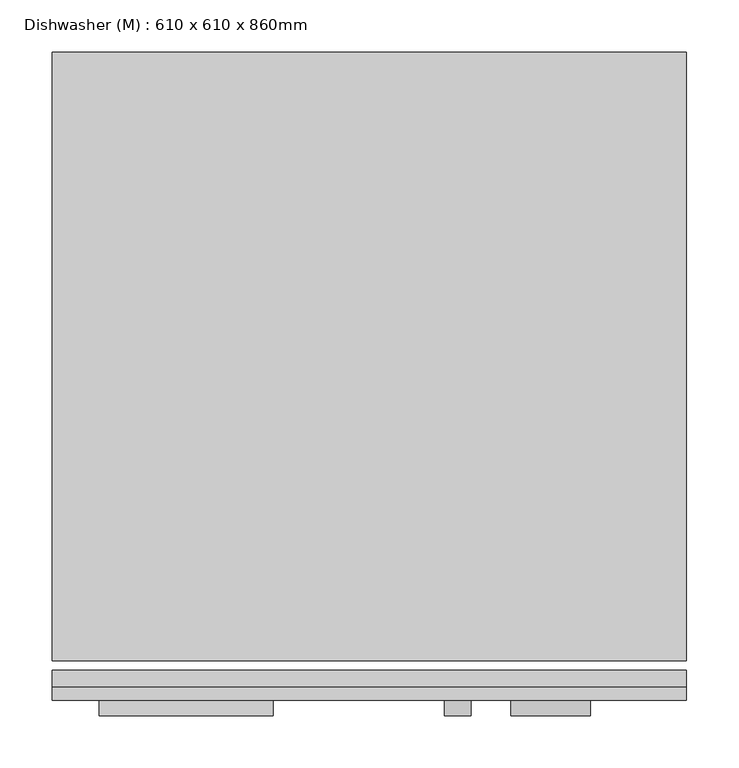
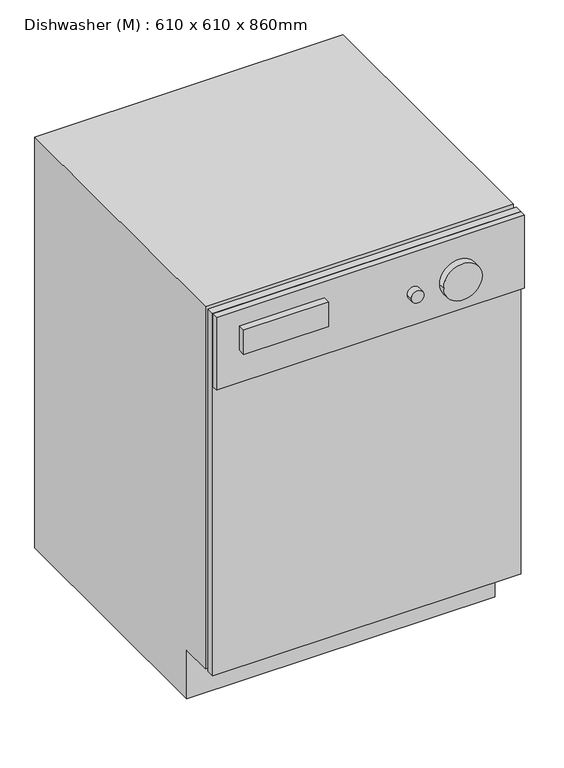
"""IFC4 building model written with IfcOpenShell, lengths in millimetres: proxy geometry, Dishwasher (M) : 610 x 610 x 860mm."""

from ifc_helpers import new_model, si_unit, point, frame, frame_2d, origin, place, context, project, spatial, polyline, circle_curve, trimmed, segment, composite_curve, outline, extrude, source, transform, mapped, element, save


def dishwasher_m_610_x_610_x_860mm_47db8dec(model_context):
    return source(origin(), model_context, "Body", "SweptSolid", [
        extrude(outline(polyline([(687.5174685, -38.3504352), (77.5174685, -38.3504352), (77.5174685, -22.4754352), (687.5174685, -22.4754352), (687.5174685, -38.3504352)])), frame((0.0, 0.0, 101.6), z_axis=(0.0, 0.0, 1.0), x_axis=(1.0, 0.0, 0.0)), (0.0, 0.0, 1.0), 758.4),
        extrude(outline(polyline([(687.5174685, -38.3504352), (687.5174685, -51.0504352), (77.5174685, -51.0504352), (77.5174685, -38.3504352), (687.5174685, -38.3504352)])), frame((0.0, 0.0, 707.6), z_axis=(0.0, 0.0, 1.0), x_axis=(1.0, 0.0, 0.0)), (0.0, 0.0, 1.0), 152.4),
        extrude(outline(polyline([(571.6495648, 0.0), (50.5495648, 0.0), (50.5495648, 101.6), (-12.9504352, 101.6), (-12.9504352, 860.0), (571.6495648, 860.0), (571.6495648, 0.0)])), frame((77.5174685, 0.0, 0.0), z_axis=(1.0, 0.0, 0.0), x_axis=(0.0, 1.0, 0.0)), (0.0, 0.0, 1.0), 610.0),
        extrude(outline(polyline([(290.2347603, -66.0504352), (122.8347603, -66.0504352), (122.8347603, -51.0504352), (290.2347603, -51.0504352), (290.2347603, -66.0504352)])), frame((0.0, 0.0, 775.6663551), z_axis=(0.0, 0.0, 1.0), x_axis=(1.0, 0.0, 0.0)), (0.0, 0.0, 1.0), 50.8),
        extrude(outline(composite_curve([segment(trimmed(circle_curve(frame_2d((775.6663551, 467.3393328)), 12.7), [point((775.6663551, 480.0393328))], [point((775.6663551, 454.6393328))], False, "CARTESIAN"), True, "CONTINUOUS"), segment(trimmed(circle_curve(frame_2d((775.6663551, 467.3393328)), 12.7), [point((775.6663551, 454.6393328))], [point((775.6663551, 480.0393328))], False, "CARTESIAN"), True, "CONTINUOUS")], self_intersect=False)), frame((0.0, -66.0504352, 0.0), z_axis=(0.0, 1.0, 0.0), x_axis=(0.0, 0.0, 1.0)), (0.0, 0.0, 1.0), 15.0),
        extrude(outline(composite_curve([segment(trimmed(circle_curve(frame_2d((775.6663551, 556.7855874)), 38.1), [point((775.6663551, 594.8855874))], [point((775.6663551, 518.6855874))], False, "CARTESIAN"), True, "CONTINUOUS"), segment(trimmed(circle_curve(frame_2d((775.6663551, 556.7855874)), 38.1), [point((775.6663551, 518.6855874))], [point((775.6663551, 594.8855874))], False, "CARTESIAN"), True, "CONTINUOUS")], self_intersect=False)), frame((0.0, -66.0504352, 0.0), z_axis=(0.0, 1.0, 0.0), x_axis=(0.0, 0.0, 1.0)), (0.0, 0.0, 1.0), 15.0),
    ])


if __name__ == "__main__":
    model = new_model("IFC4")
    model_context = context("Model", 3, world=origin())
    ifc_project = project(units=[si_unit("LENGTHUNIT", "METRE", prefix="MILLI")], contexts=[model_context])
    site = spatial("IfcSite", under=ifc_project)
    building = spatial("IfcBuilding", under=site)
    placement = place(None, origin())
    dishwasher_m_610_x_610_x_860mm_shape = dishwasher_m_610_x_610_x_860mm_47db8dec(model_context)
    element("IfcBuildingElementProxy", 1, Name="Dishwasher (M) : 610 x 610 x 860mm", ObjectType="Dishwasher (M) : 610 x 610 x 860mm", at=placement, inside=building, context=model_context, shape_type="MappedRepresentation", body=[
        mapped(dishwasher_m_610_x_610_x_860mm_shape, transform((0.0, 0.0, 0.0), x_axis=(1.0, 0.0, 0.0), y_axis=(0.0, 1.0, 0.0), z_axis=(0.0, 0.0, 1.0))),
    ])
    save(model, "model.ifc")

# Revit data of these elements
# Type "Dishwasher (M) : 610 x 610 x 860mm"
#   Label = "DW"
#   Depth = 2' - 0.01575"
#   Height = 2' - 9.85827"
#   Width = 2' - 0.01575"
#   Dishwasher Material = Metal - Paint Finish - Ivory,Glossy
#   Panel Face Material = Plastic - Black
#   Default Elevation = 0
# Element 1 (IfcBuildingElementProxy, "Dishwasher (M) : 610 x 610 x 860mm")
#   Materials on its faces: "Metal - Paint Finish - Ivory,Glossy", "Plastic - Black"
# Materials
#   "Metal - Paint Finish - Ivory,Glossy": colour RGB 247 247 239, transparency 0
#   "Plastic - Black": colour RGB 0 0 0, transparency 0.7
